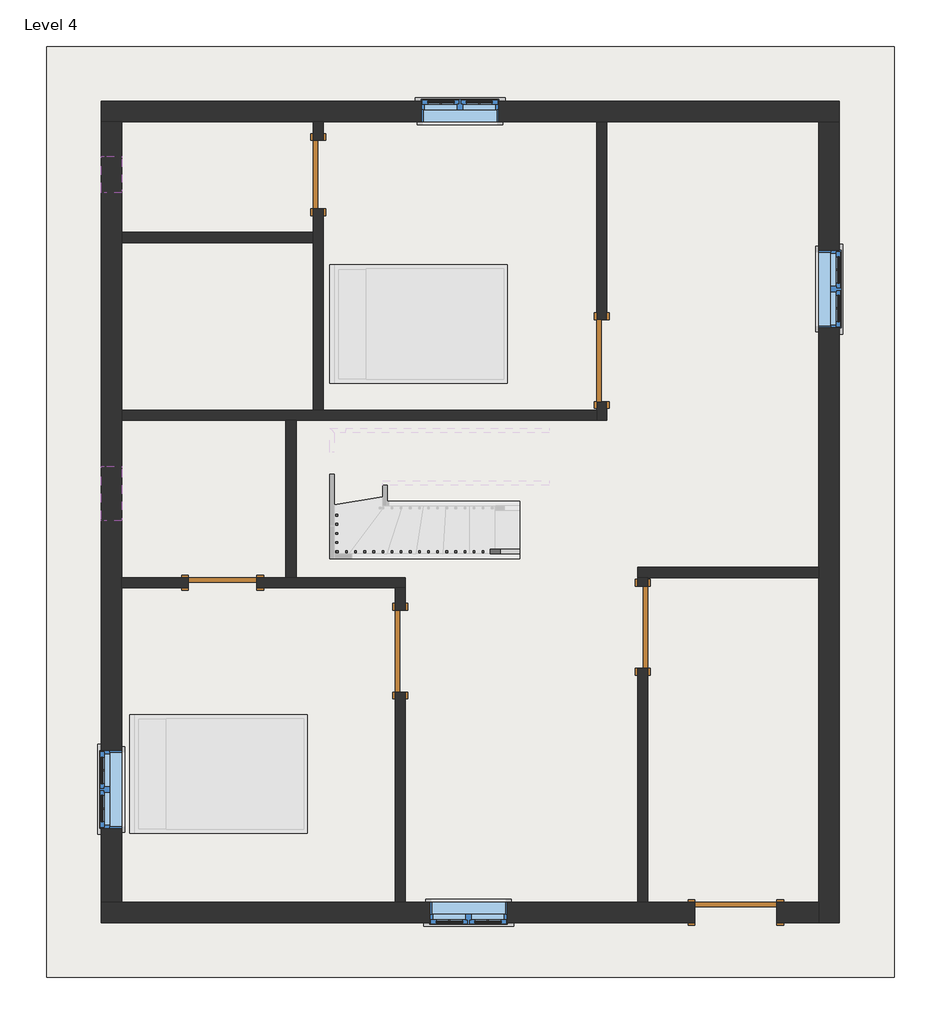
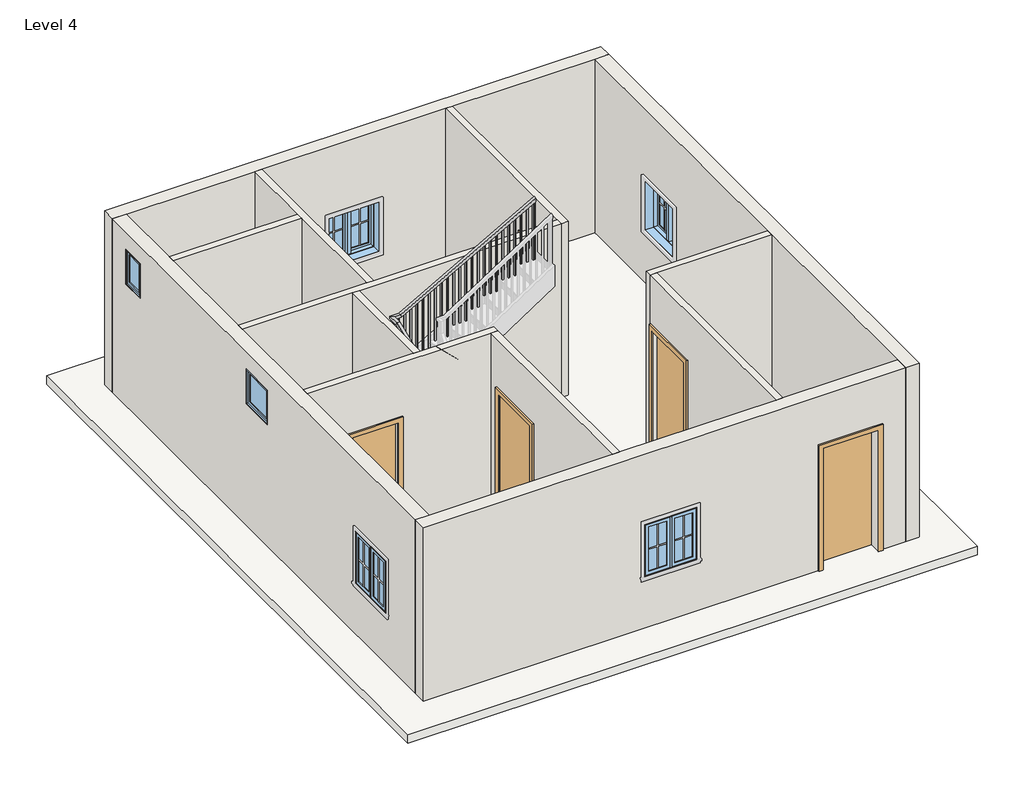
# One storey, part 1 of 2: 13 walls, 6 doors, 6 windows, 1 railing, 1 roof.
"""IFC4 building model written with IfcOpenShell, lengths in millimetres."""

from ifc_helpers import new_model, si_unit, frame, origin, place, context, project, spatial, polyline, outline, extrude, faceted_brep, transform, mapped, element, save
from components import door_d8f5dbb5, door_f2b275c1, door_305aa2a5, door_e5f9f3c4, door_0ca8825f, window_aa618e30, window_80340324, window_339605e1

model = new_model("IFC4")

# Units and contexts
model_context = context("Model", 3, world=origin())
ifc_project = project(units=[si_unit("LENGTHUNIT", "METRE", prefix="MILLI")], contexts=[model_context])

# Site, building, storey
site = spatial("IfcSite", under=ifc_project)
building = spatial("IfcBuilding", under=site)
storey = spatial("IfcBuildingStorey", under=building, Name="Level 4", Elevation=6400.8)

# Doors
placement = place(None, origin())
door_shape = door_d8f5dbb5(model_context)
element("IfcDoor", 1, ObjectType="Single-Flush : 30\" x 80\"", at=placement, inside=storey, context=model_context, shape_type="MappedRepresentation", body=[
    mapped(door_shape, transform((-2510.1648498, 3958.5558073, 6400.8), x_axis=(0.0, 1.0, 0.0), y_axis=(-1.0, 0.0, 0.0), z_axis=(0.0, 0.0, 1.0))),
])
door_2_shape = door_f2b275c1(model_context)
element("IfcDoor", 2, ObjectType="Single-Flush : 30\" x 80\"", at=placement, inside=storey, context=model_context, shape_type="MappedRepresentation", body=[
    mapped(door_2_shape, transform((-3576.9648498, -592.8066927, 6400.8), x_axis=(-1.0, 0.0, 0.0), y_axis=(0.0, -1.0, 0.0), z_axis=(0.0, 0.0, 1.0))),
])
door_3_shape = door_305aa2a5(model_context)
element("IfcDoor", 3, ObjectType="Single-Flush : 36\" x 84\"", at=placement, inside=storey, context=model_context, shape_type="MappedRepresentation", body=[
    mapped(door_3_shape, transform((652.1351502, 1883.6933073, 6400.8), x_axis=(0.0, -1.0, 0.0), y_axis=(1.0, 0.0, 0.0), z_axis=(0.0, 0.0, 1.0))),
])
element("IfcDoor", 4, ObjectType="Single-Flush : 36\" x 84\"", at=placement, inside=storey, context=model_context, shape_type="MappedRepresentation", body=[
    mapped(door_3_shape, transform((1109.3351502, -1088.1066927, 6400.8), x_axis=(0.0, 1.0, 0.0), y_axis=(-1.0, 0.0, 0.0), z_axis=(0.0, 0.0, 1.0))),
])
door_4_shape = door_e5f9f3c4(model_context)
element("IfcDoor", 5, ObjectType="Single-Flush : 36\" x 84\"", at=placement, inside=storey, context=model_context, shape_type="MappedRepresentation", body=[
    mapped(door_4_shape, transform((-1595.7648498, -1354.8066927, 6400.8), x_axis=(0.0, 1.0, 0.0), y_axis=(-1.0, 0.0, 0.0), z_axis=(0.0, 0.0, 1.0))),
])
door_5_shape = door_0ca8825f(model_context)
element("IfcDoor", 6, ObjectType="Single-Flush : 36\" x 84\"", at=placement, inside=storey, context=model_context, shape_type="MappedRepresentation", body=[
    mapped(door_5_shape, transform((2147.5601502, -4269.4566927, 6400.8), x_axis=(1.0, 0.0, 0.0), y_axis=(0.0, 1.0, 0.0), z_axis=(0.0, 0.0, 1.0))),
])

# Railing
element("IfcRailing", 7, ObjectType="Handrail - Rectangular", at=placement, inside=storey, context=model_context, shape_type="SolidModel", body=[
    faceted_brep([(-264.8831579, -271.8029286, 7484.5333333), (-264.8831579, -271.8029286, 7426.9518622), (-264.8831579, -221.0029286, 7426.9518622), (-264.8831579, -221.0029286, 7484.5333333), (-2203.3957557, -271.8029286, 8519.066441), (-2216.1029055, -271.8029286, 8468.266441), (-2216.1029055, -221.0029286, 8468.266441), (-2203.3957557, -221.0029286, 8519.066441), (-2328.8610857, -271.8029286, 8519.066441), (-2328.8610857, -271.8029286, 8468.266441), (-2278.0610857, -221.0029286, 8468.266441), (-2278.0610857, -221.0029286, 8519.066441), (-2328.8610857, -117.3180853, 8519.066441), (-2328.8610857, -107.2249429, 8468.266441), (-2278.0610857, -107.2249429, 8468.266441), (-2278.0610857, -117.3180853, 8519.066441), (-2328.8610857, 889.2076495, 8935.4648193), (-2328.8610857, 899.300792, 8884.6648193), (-2278.0610857, 899.300792, 8884.6648193), (-2278.0610857, 889.2076495, 8935.4648193), (-2328.8610857, 1080.0895433, 8935.4648193), (-2328.8610857, 1080.0895433, 8884.6648193), (-2278.0610857, 1029.2895433, 8884.6648193), (-2278.0610857, 1029.2895433, 8935.4648193), (-2181.3423106, 1080.0895433, 8935.4648193), (-2168.0744201, 1080.0895433, 8884.6648193), (-2168.0744201, 1029.2895433, 8884.6648193), (-2181.3423106, 1029.2895433, 8935.4648193), (63.4034409, 1080.0895433, 10193.8666667), (63.4034409, 1029.2895433, 10193.8666667), (63.4034409, 1029.2895433, 10135.6287027), (63.4034409, 1080.0895433, 10135.6287027)], [[[0, 1, 2, 3]], [[1, 0, 4, 5]], [[2, 1, 5, 6]], [[3, 2, 6, 7]], [[0, 3, 7, 4]], [[5, 4, 8, 9]], [[6, 5, 9, 10]], [[7, 6, 10, 11]], [[4, 7, 11, 8]], [[9, 8, 12, 13]], [[10, 9, 13, 14]], [[11, 10, 14, 15]], [[8, 11, 15, 12]], [[13, 12, 16, 17]], [[14, 13, 17, 18]], [[15, 14, 18, 19]], [[12, 15, 19, 16]], [[17, 16, 20, 21]], [[18, 17, 21, 22]], [[19, 18, 22, 23]], [[16, 19, 23, 20]], [[21, 20, 24, 25]], [[22, 21, 25, 26]], [[23, 22, 26, 27]], [[20, 23, 27, 24]], [[28, 29, 30, 31]], [[25, 24, 28, 31]], [[26, 25, 31, 30]], [[27, 26, 30, 29]], [[24, 27, 29, 28]]]),
    extrude(outline(polyline([(10113.4348603, 23.8139143), (9110.1333333, 23.8139143), (9110.1333333, 42.8639143), (10124.1142681, 42.8639143), (10113.4348603, 23.8139143)])), frame((0.0, 1045.1645433, 0.0), z_axis=(0.0, 1.0, 0.0), x_axis=(0.0, 0.0, 1.0)), (0.0, 0.0, 1.0), 19.05),
    extrude(outline(polyline([(10056.478019, -77.7860857), (9110.1333333, -77.7860857), (9110.1333333, -58.7360857), (10067.1574267, -58.7360857), (10056.478019, -77.7860857)])), frame((0.0, 1045.1645433, 0.0), z_axis=(0.0, 1.0, 0.0), x_axis=(0.0, 0.0, 1.0)), (0.0, 0.0, 1.0), 19.05),
    extrude(outline(polyline([(9999.5211776, -179.3860857), (9110.1333333, -179.3860857), (9110.1333333, -160.3360857), (10010.2005853, -160.3360857), (9999.5211776, -179.3860857)])), frame((0.0, 1045.1645433, 0.0), z_axis=(0.0, 1.0, 0.0), x_axis=(0.0, 0.0, 1.0)), (0.0, 0.0, 1.0), 19.05),
    extrude(outline(polyline([(9942.5643362, -280.9860857), (8940.8, -280.9860857), (8940.8, -261.9360857), (9953.243744, -261.9360857), (9942.5643362, -280.9860857)])), frame((0.0, 1045.1645433, 0.0), z_axis=(0.0, 1.0, 0.0), x_axis=(0.0, 0.0, 1.0)), (0.0, 0.0, 1.0), 19.05),
    extrude(outline(polyline([(9885.6074948, -382.5860857), (8940.8, -382.5860857), (8940.8, -363.5360857), (9896.2869026, -363.5360857), (9885.6074948, -382.5860857)])), frame((0.0, 1045.1645433, 0.0), z_axis=(0.0, 1.0, 0.0), x_axis=(0.0, 0.0, 1.0)), (0.0, 0.0, 1.0), 19.05),
    extrude(outline(polyline([(9828.6506535, -484.1860857), (8940.8, -484.1860857), (8940.8, -465.1360857), (9839.3300612, -465.1360857), (9828.6506535, -484.1860857)])), frame((0.0, 1045.1645433, 0.0), z_axis=(0.0, 1.0, 0.0), x_axis=(0.0, 0.0, 1.0)), (0.0, 0.0, 1.0), 19.05),
    extrude(outline(polyline([(9771.6938121, -585.7860857), (8771.4666667, -585.7860857), (8771.4666667, -566.7360857), (9782.3732198, -566.7360857), (9771.6938121, -585.7860857)])), frame((0.0, 1045.1645433, 0.0), z_axis=(0.0, 1.0, 0.0), x_axis=(0.0, 0.0, 1.0)), (0.0, 0.0, 1.0), 19.05),
    extrude(outline(polyline([(9714.7369707, -687.3860857), (8771.4666667, -687.3860857), (8771.4666667, -668.3360857), (9725.4163785, -668.3360857), (9714.7369707, -687.3860857)])), frame((0.0, 1045.1645433, 0.0), z_axis=(0.0, 1.0, 0.0), x_axis=(0.0, 0.0, 1.0)), (0.0, 0.0, 1.0), 19.05),
    extrude(outline(polyline([(9657.7801293, -788.9860857), (8771.4666667, -788.9860857), (8771.4666667, -769.9360857), (9668.4595371, -769.9360857), (9657.7801293, -788.9860857)])), frame((0.0, 1045.1645433, 0.0), z_axis=(0.0, 1.0, 0.0), x_axis=(0.0, 0.0, 1.0)), (0.0, 0.0, 1.0), 19.05),
    extrude(outline(polyline([(9600.823288, -890.5860857), (8602.1333333, -890.5860857), (8602.1333333, -871.5360857), (9611.5026957, -871.5360857), (9600.823288, -890.5860857)])), frame((0.0, 1045.1645433, 0.0), z_axis=(0.0, 1.0, 0.0), x_axis=(0.0, 0.0, 1.0)), (0.0, 0.0, 1.0), 19.05),
    extrude(outline(polyline([(9543.8664466, -992.1860857), (8602.1333333, -992.1860857), (8602.1333333, -973.1360857), (9554.5458543, -973.1360857), (9543.8664466, -992.1860857)])), frame((0.0, 1045.1645433, 0.0), z_axis=(0.0, 1.0, 0.0), x_axis=(0.0, 0.0, 1.0)), (0.0, 0.0, 1.0), 19.05),
    extrude(outline(polyline([(9486.9096052, -1093.7860857), (8432.8, -1093.7860857), (8432.8, -1074.7360857), (9497.589013, -1074.7360857), (9486.9096052, -1093.7860857)])), frame((0.0, 1045.1645433, 0.0), z_axis=(0.0, 1.0, 0.0), x_axis=(0.0, 0.0, 1.0)), (0.0, 0.0, 1.0), 19.05),
    extrude(outline(polyline([(9429.9527638, -1195.3860857), (8432.8, -1195.3860857), (8432.8, -1176.3360857), (9440.6321716, -1176.3360857), (9429.9527638, -1195.3860857)])), frame((0.0, 1045.1645433, 0.0), z_axis=(0.0, 1.0, 0.0), x_axis=(0.0, 0.0, 1.0)), (0.0, 0.0, 1.0), 19.05),
    extrude(outline(polyline([(9372.9959225, -1296.9860857), (8432.8, -1296.9860857), (8432.8, -1277.9360857), (9383.6753302, -1277.9360857), (9372.9959225, -1296.9860857)])), frame((0.0, 1045.1645433, 0.0), z_axis=(0.0, 1.0, 0.0), x_axis=(0.0, 0.0, 1.0)), (0.0, 0.0, 1.0), 19.05),
    extrude(outline(polyline([(9316.0390811, -1398.5860857), (8263.4666667, -1398.5860857), (8263.4666667, -1379.5360857), (9326.7184889, -1379.5360857), (9316.0390811, -1398.5860857)])), frame((0.0, 1045.1645433, 0.0), z_axis=(0.0, 1.0, 0.0), x_axis=(0.0, 0.0, 1.0)), (0.0, 0.0, 1.0), 19.05),
    extrude(outline(polyline([(9259.0822397, -1500.1860857), (8263.4666667, -1500.1860857), (8263.4666667, -1481.1360857), (9269.7616475, -1481.1360857), (9259.0822397, -1500.1860857)])), frame((0.0, 1045.1645433, 0.0), z_axis=(0.0, 1.0, 0.0), x_axis=(0.0, 0.0, 1.0)), (0.0, 0.0, 1.0), 19.05),
    extrude(outline(polyline([(9202.1253983, -1601.7860857), (8263.4666667, -1601.7860857), (8263.4666667, -1582.7360857), (9212.8048061, -1582.7360857), (9202.1253983, -1601.7860857)])), frame((0.0, 1045.1645433, 0.0), z_axis=(0.0, 1.0, 0.0), x_axis=(0.0, 0.0, 1.0)), (0.0, 0.0, 1.0), 19.05),
    extrude(outline(polyline([(9145.168557, -1703.3860857), (8094.1333333, -1703.3860857), (8094.1333333, -1684.3360857), (9155.8479647, -1684.3360857), (9145.168557, -1703.3860857)])), frame((0.0, 1045.1645433, 0.0), z_axis=(0.0, 1.0, 0.0), x_axis=(0.0, 0.0, 1.0)), (0.0, 0.0, 1.0), 19.05),
    extrude(outline(polyline([(9088.2117156, -1804.9860857), (8094.1333333, -1804.9860857), (8094.1333333, -1785.9360857), (9098.8911234, -1785.9360857), (9088.2117156, -1804.9860857)])), frame((0.0, 1045.1645433, 0.0), z_axis=(0.0, 1.0, 0.0), x_axis=(0.0, 0.0, 1.0)), (0.0, 0.0, 1.0), 19.05),
    extrude(outline(polyline([(9031.2548742, -1906.5860857), (8094.1333333, -1906.5860857), (8094.1333333, -1887.5360857), (9041.934282, -1887.5360857), (9031.2548742, -1906.5860857)])), frame((0.0, 1045.1645433, 0.0), z_axis=(0.0, 1.0, 0.0), x_axis=(0.0, 0.0, 1.0)), (0.0, 0.0, 1.0), 19.05),
    extrude(outline(polyline([(8974.2980329, -2008.1860857), (8094.1333333, -2008.1860857), (8094.1333333, -1989.1360857), (8984.9774406, -1989.1360857), (8974.2980329, -2008.1860857)])), frame((0.0, 1045.1645433, 0.0), z_axis=(0.0, 1.0, 0.0), x_axis=(0.0, 0.0, 1.0)), (0.0, 0.0, 1.0), 19.05),
    extrude(outline(polyline([(8917.3411915, -2109.7860857), (7924.8, -2109.7860857), (7924.8, -2090.7360857), (8928.0205992, -2090.7360857), (8917.3411915, -2109.7860857)])), frame((0.0, 1045.1645433, 0.0), z_axis=(0.0, 1.0, 0.0), x_axis=(0.0, 0.0, 1.0)), (0.0, 0.0, 1.0), 19.05),
    extrude(outline(polyline([(-2211.3860857, 1064.2145433), (-2192.3360857, 1064.2145433), (-2192.3360857, 1045.1645433), (-2211.3860857, 1045.1645433), (-2211.3860857, 1064.2145433)])), frame((0.0, 0.0, 7924.8), z_axis=(0.0, 0.0, 1.0), x_axis=(1.0, 0.0, 0.0)), (0.0, 0.0, 1.0), 959.8648193),
    extrude(outline(polyline([(-2312.9860857, 963.2720714), (-2312.9860857, 982.3220714), (-2293.9360857, 982.3220714), (-2293.9360857, 963.2720714), (-2312.9860857, 963.2720714)])), frame((0.0, 0.0, 7924.8), z_axis=(0.0, 0.0, 1.0), x_axis=(1.0, 0.0, 0.0)), (0.0, 0.0, 1.0), 959.8648193),
    extrude(outline(polyline([(880.7220714, 8876.9788269), (880.7220714, 7924.8), (861.6720714, 7924.8), (861.6720714, 8869.0978669), (880.7220714, 8876.9788269)])), frame((-2312.9860857, 0.0, 0.0), z_axis=(1.0, 0.0, 0.0), x_axis=(0.0, 1.0, 0.0)), (0.0, 0.0, 1.0), 19.05),
    extrude(outline(polyline([(779.1220714, 8834.94704), (779.1220714, 7924.8), (760.0720714, 7924.8), (760.0720714, 8827.0660799), (779.1220714, 8834.94704)])), frame((-2312.9860857, 0.0, 0.0), z_axis=(1.0, 0.0, 0.0), x_axis=(0.0, 1.0, 0.0)), (0.0, 0.0, 1.0), 19.05),
    extrude(outline(polyline([(677.5220714, 8792.915253), (677.5220714, 7924.8), (658.4720714, 7924.8), (658.4720714, 8785.034293), (677.5220714, 8792.915253)])), frame((-2312.9860857, 0.0, 0.0), z_axis=(1.0, 0.0, 0.0), x_axis=(0.0, 1.0, 0.0)), (0.0, 0.0, 1.0), 19.05),
    extrude(outline(polyline([(575.9220714, 8750.8834661), (575.9220714, 7755.4666667), (556.8720714, 7755.4666667), (556.8720714, 8743.002506), (575.9220714, 8750.8834661)])), frame((-2312.9860857, 0.0, 0.0), z_axis=(1.0, 0.0, 0.0), x_axis=(0.0, 1.0, 0.0)), (0.0, 0.0, 1.0), 19.05),
    extrude(outline(polyline([(474.3220714, 8708.8516792), (474.3220714, 7755.4666667), (455.2720714, 7755.4666667), (455.2720714, 8700.9707191), (474.3220714, 8708.8516792)])), frame((-2312.9860857, 0.0, 0.0), z_axis=(1.0, 0.0, 0.0), x_axis=(0.0, 1.0, 0.0)), (0.0, 0.0, 1.0), 19.05),
    extrude(outline(polyline([(372.7220714, 8666.8198922), (372.7220714, 7755.4666667), (353.6720714, 7755.4666667), (353.6720714, 8658.9389322), (372.7220714, 8666.8198922)])), frame((-2312.9860857, 0.0, 0.0), z_axis=(1.0, 0.0, 0.0), x_axis=(0.0, 1.0, 0.0)), (0.0, 0.0, 1.0), 19.05),
    extrude(outline(polyline([(271.1220714, 8624.7881053), (271.1220714, 7755.4666667), (252.0720714, 7755.4666667), (252.0720714, 8616.9071452), (271.1220714, 8624.7881053)])), frame((-2312.9860857, 0.0, 0.0), z_axis=(1.0, 0.0, 0.0), x_axis=(0.0, 1.0, 0.0)), (0.0, 0.0, 1.0), 19.05),
    extrude(outline(polyline([(169.5220714, 8582.7563183), (169.5220714, 7586.1333333), (150.4720714, 7586.1333333), (150.4720714, 8574.8753583), (169.5220714, 8582.7563183)])), frame((-2312.9860857, 0.0, 0.0), z_axis=(1.0, 0.0, 0.0), x_axis=(0.0, 1.0, 0.0)), (0.0, 0.0, 1.0), 19.05),
    extrude(outline(polyline([(67.9220714, 8540.7245314), (67.9220714, 7586.1333333), (48.8720714, 7586.1333333), (48.8720714, 8532.8435714), (67.9220714, 8540.7245314)])), frame((-2312.9860857, 0.0, 0.0), z_axis=(1.0, 0.0, 0.0), x_axis=(0.0, 1.0, 0.0)), (0.0, 0.0, 1.0), 19.05),
    extrude(outline(polyline([(-33.6779286, 8498.6927445), (-33.6779286, 7586.1333333), (-52.7279286, 7586.1333333), (-52.7279286, 8490.8117844), (-33.6779286, 8498.6927445)])), frame((-2312.9860857, 0.0, 0.0), z_axis=(1.0, 0.0, 0.0), x_axis=(0.0, 1.0, 0.0)), (0.0, 0.0, 1.0), 19.05),
    extrude(outline(polyline([(-2312.9860857, -154.3279286), (-2312.9860857, -135.2779286), (-2293.9360857, -135.2779286), (-2293.9360857, -154.3279286), (-2312.9860857, -154.3279286)])), frame((0.0, 0.0, 7586.1333333), z_axis=(0.0, 0.0, 1.0), x_axis=(1.0, 0.0, 0.0)), (0.0, 0.0, 1.0), 882.1331077),
    extrude(outline(polyline([(-2287.3581579, -255.9279286), (-2306.4081579, -255.9279286), (-2306.4081579, -236.8779286), (-2287.3581579, -236.8779286), (-2287.3581579, -255.9279286)])), frame((0.0, 0.0, 7586.1333333), z_axis=(0.0, 0.0, 1.0), x_axis=(1.0, 0.0, 0.0)), (0.0, 0.0, 1.0), 882.1331077),
    extrude(outline(polyline([(8462.2387317, -2204.8081579), (7586.1333333, -2204.8081579), (7586.1333333, -2185.7581579), (8452.0722486, -2185.7581579), (8462.2387317, -2204.8081579)])), frame((0.0, -255.9279286, 0.0), z_axis=(0.0, 1.0, 0.0), x_axis=(0.0, 0.0, 1.0)), (0.0, 0.0, 1.0), 19.05),
    extrude(outline(polyline([(8408.0174882, -2103.2081579), (7416.8, -2103.2081579), (7416.8, -2084.1581579), (8397.851005, -2084.1581579), (8408.0174882, -2103.2081579)])), frame((0.0, -255.9279286, 0.0), z_axis=(0.0, 1.0, 0.0), x_axis=(0.0, 0.0, 1.0)), (0.0, 0.0, 1.0), 19.05),
    extrude(outline(polyline([(8353.7962446, -2001.6081579), (7416.8, -2001.6081579), (7416.8, -1982.5581579), (8343.6297614, -1982.5581579), (8353.7962446, -2001.6081579)])), frame((0.0, -255.9279286, 0.0), z_axis=(0.0, 1.0, 0.0), x_axis=(0.0, 0.0, 1.0)), (0.0, 0.0, 1.0), 19.05),
    extrude(outline(polyline([(8299.575001, -1900.0081579), (7416.8, -1900.0081579), (7416.8, -1880.9581579), (8289.4085178, -1880.9581579), (8299.575001, -1900.0081579)])), frame((0.0, -255.9279286, 0.0), z_axis=(0.0, 1.0, 0.0), x_axis=(0.0, 0.0, 1.0)), (0.0, 0.0, 1.0), 19.05),
    extrude(outline(polyline([(8245.3537574, -1798.4081579), (7416.8, -1798.4081579), (7416.8, -1779.3581579), (8235.1872743, -1779.3581579), (8245.3537574, -1798.4081579)])), frame((0.0, -255.9279286, 0.0), z_axis=(0.0, 1.0, 0.0), x_axis=(0.0, 0.0, 1.0)), (0.0, 0.0, 1.0), 19.05),
    extrude(outline(polyline([(8191.1325139, -1696.8081579), (7247.4666667, -1696.8081579), (7247.4666667, -1677.7581579), (8180.9660307, -1677.7581579), (8191.1325139, -1696.8081579)])), frame((0.0, -255.9279286, 0.0), z_axis=(0.0, 1.0, 0.0), x_axis=(0.0, 0.0, 1.0)), (0.0, 0.0, 1.0), 19.05),
    extrude(outline(polyline([(8136.9112703, -1595.2081579), (7247.4666667, -1595.2081579), (7247.4666667, -1576.1581579), (8126.7447871, -1576.1581579), (8136.9112703, -1595.2081579)])), frame((0.0, -255.9279286, 0.0), z_axis=(0.0, 1.0, 0.0), x_axis=(0.0, 0.0, 1.0)), (0.0, 0.0, 1.0), 19.05),
    extrude(outline(polyline([(8082.6900267, -1493.6081579), (7247.4666667, -1493.6081579), (7247.4666667, -1474.5581579), (8072.5235435, -1474.5581579), (8082.6900267, -1493.6081579)])), frame((0.0, -255.9279286, 0.0), z_axis=(0.0, 1.0, 0.0), x_axis=(0.0, 0.0, 1.0)), (0.0, 0.0, 1.0), 19.05),
    extrude(outline(polyline([(8028.4687831, -1392.0081579), (7078.1333333, -1392.0081579), (7078.1333333, -1372.9581579), (8018.3023, -1372.9581579), (8028.4687831, -1392.0081579)])), frame((0.0, -255.9279286, 0.0), z_axis=(0.0, 1.0, 0.0), x_axis=(0.0, 0.0, 1.0)), (0.0, 0.0, 1.0), 19.05),
    extrude(outline(polyline([(7974.2475396, -1290.4081579), (7078.1333333, -1290.4081579), (7078.1333333, -1271.3581579), (7964.0810564, -1271.3581579), (7974.2475396, -1290.4081579)])), frame((0.0, -255.9279286, 0.0), z_axis=(0.0, 1.0, 0.0), x_axis=(0.0, 0.0, 1.0)), (0.0, 0.0, 1.0), 19.05),
    extrude(outline(polyline([(7920.026296, -1188.8081579), (7078.1333333, -1188.8081579), (7078.1333333, -1169.7581579), (7909.8598128, -1169.7581579), (7920.026296, -1188.8081579)])), frame((0.0, -255.9279286, 0.0), z_axis=(0.0, 1.0, 0.0), x_axis=(0.0, 0.0, 1.0)), (0.0, 0.0, 1.0), 19.05),
    extrude(outline(polyline([(7865.8050524, -1087.2081579), (6908.8, -1087.2081579), (6908.8, -1068.1581579), (7855.6385692, -1068.1581579), (7865.8050524, -1087.2081579)])), frame((0.0, -255.9279286, 0.0), z_axis=(0.0, 1.0, 0.0), x_axis=(0.0, 0.0, 1.0)), (0.0, 0.0, 1.0), 19.05),
    extrude(outline(polyline([(7811.5838088, -985.6081579), (6908.8, -985.6081579), (6908.8, -966.5581579), (7801.4173257, -966.5581579), (7811.5838088, -985.6081579)])), frame((0.0, -255.9279286, 0.0), z_axis=(0.0, 1.0, 0.0), x_axis=(0.0, 0.0, 1.0)), (0.0, 0.0, 1.0), 19.05),
    extrude(outline(polyline([(7757.3625653, -884.0081579), (6908.8, -884.0081579), (6908.8, -864.9581579), (7747.1960821, -864.9581579), (7757.3625653, -884.0081579)])), frame((0.0, -255.9279286, 0.0), z_axis=(0.0, 1.0, 0.0), x_axis=(0.0, 0.0, 1.0)), (0.0, 0.0, 1.0), 19.05),
    extrude(outline(polyline([(7703.1413217, -782.4081579), (6739.4666667, -782.4081579), (6739.4666667, -763.3581579), (7692.9748385, -763.3581579), (7703.1413217, -782.4081579)])), frame((0.0, -255.9279286, 0.0), z_axis=(0.0, 1.0, 0.0), x_axis=(0.0, 0.0, 1.0)), (0.0, 0.0, 1.0), 19.05),
    extrude(outline(polyline([(7648.9200781, -680.8081579), (6739.4666667, -680.8081579), (6739.4666667, -661.7581579), (7638.7535949, -661.7581579), (7648.9200781, -680.8081579)])), frame((0.0, -255.9279286, 0.0), z_axis=(0.0, 1.0, 0.0), x_axis=(0.0, 0.0, 1.0)), (0.0, 0.0, 1.0), 19.05),
    extrude(outline(polyline([(7594.6988345, -579.2081579), (6739.4666667, -579.2081579), (6739.4666667, -560.1581579), (7584.5323514, -560.1581579), (7594.6988345, -579.2081579)])), frame((0.0, -255.9279286, 0.0), z_axis=(0.0, 1.0, 0.0), x_axis=(0.0, 0.0, 1.0)), (0.0, 0.0, 1.0), 19.05),
    extrude(outline(polyline([(7540.477591, -477.6081579), (6570.1333333, -477.6081579), (6570.1333333, -458.5581579), (7530.3111078, -458.5581579), (7540.477591, -477.6081579)])), frame((0.0, -255.9279286, 0.0), z_axis=(0.0, 1.0, 0.0), x_axis=(0.0, 0.0, 1.0)), (0.0, 0.0, 1.0), 19.05),
    extrude(outline(polyline([(7486.2563474, -376.0081579), (6570.1333333, -376.0081579), (6570.1333333, -356.9581579), (7476.0898642, -356.9581579), (7486.2563474, -376.0081579)])), frame((0.0, -255.9279286, 0.0), z_axis=(0.0, 1.0, 0.0), x_axis=(0.0, 0.0, 1.0)), (0.0, 0.0, 1.0), 19.05),
    extrude(outline(polyline([(-2312.9860857, 1045.1645433), (-2312.9860857, 1064.2145433), (-2293.9360857, 1064.2145433), (-2293.9360857, 1045.1645433), (-2312.9860857, 1045.1645433)])), frame((0.0, 0.0, 7924.8), z_axis=(0.0, 0.0, 1.0), x_axis=(1.0, 0.0, 0.0)), (0.0, 0.0, 1.0), 959.8648193),
    extrude(outline(polyline([(-2293.9360857, -255.9279286), (-2312.9860857, -255.9279286), (-2312.9860857, -236.8779286), (-2293.9360857, -236.8779286), (-2293.9360857, -255.9279286)])), frame((0.0, 0.0, 7586.1333333), z_axis=(0.0, 0.0, 1.0), x_axis=(1.0, 0.0, 0.0)), (0.0, 0.0, 1.0), 882.1331077),
    extrude(outline(polyline([(10124.949295, 44.3534409), (9110.1333333, 44.3534409), (9110.1333333, 63.4034409), (10135.6287027, 63.4034409), (10124.949295, 44.3534409)])), frame((0.0, 1045.1645433, 0.0), z_axis=(0.0, 1.0, 0.0), x_axis=(0.0, 0.0, 1.0)), (0.0, 0.0, 1.0), 19.05),
    extrude(outline(polyline([(7437.1183454, -283.9331579), (6570.1333333, -283.9331579), (6570.1333333, -264.8831579), (7426.9518622, -264.8831579), (7437.1183454, -283.9331579)])), frame((0.0, -255.9279286, 0.0), z_axis=(0.0, 1.0, 0.0), x_axis=(0.0, 0.0, 1.0)), (0.0, 0.0, 1.0), 19.05),
])

# Roof
element("IfcRoof", 8, ObjectType="Generic - 12\"", at=placement, inside=storey, context=model_context, shape_type="SweptSolid", body=[
    extrude(outline(polyline([(-5539.1148498, 5385.7183073), (3909.6851502, 5385.7183073), (3909.6851502, -4993.3566927), (-5539.1148498, -4993.3566927), (-5539.1148498, 5385.7183073)])), frame((0.0, 0.0, 6248.4), z_axis=(0.0, 0.0, 1.0), x_axis=(1.0, 0.0, 0.0)), (0.0, 0.0, 1.0), 152.4),
])

# Walls
element("IfcWall", 9, ObjectType="WALL4.5\"", at=placement, inside=storey, context=model_context, shape_type="SweptSolid", body=[
    extrude(outline(polyline([(-2567.3148498, 3198.1433073), (-4700.9148498, 3198.1433073), (-4700.9148498, 3312.4433073), (-2567.3148498, 3312.4433073), (-2567.3148498, 3198.1433073)])), frame((0.0, 0.0, 6400.8), z_axis=(0.0, 0.0, 1.0), x_axis=(1.0, 0.0, 0.0)), (0.0, 0.0, 1.0), 3048.0),
])
element("IfcWall", 10, ObjectType="WALL4.5\"", at=placement, inside=storey, context=model_context, shape_type="Brep", body=[
    faceted_brep([(-2567.3148498, 4547.5183073, 6400.8), (-2567.3148498, 4339.5558073, 6400.8), (-2567.3148498, 4339.5558073, 8432.8), (-2567.3148498, 3577.5558073, 8432.8), (-2567.3148498, 3577.5558073, 6400.8), (-2567.3148498, 3312.4433073, 6400.8), (-2567.3148498, 3198.1433073, 6400.8), (-2567.3148498, 1331.2433073, 6400.8), (-2567.3148498, 1331.2433073, 9448.8), (-2567.3148498, 3198.1433073, 9448.8), (-2567.3148498, 3312.4433073, 9448.8), (-2567.3148498, 4547.5183073, 9448.8), (-2453.0148498, 4339.5558073, 8432.8), (-2453.0148498, 4339.5558073, 6400.8), (-2453.0148498, 4547.5183073, 6400.8), (-2453.0148498, 4547.5183073, 9448.8), (-2453.0148498, 1331.2433073, 9448.8), (-2453.0148498, 1331.2433073, 6400.8), (-2453.0148498, 3577.5558073, 6400.8), (-2453.0148498, 3577.5558073, 8432.8)], [[[0, 1, 2, 3, 4, 5, 6, 7, 8, 9, 10, 11]], [[12, 13, 14, 15, 16, 17, 18, 19]], [[18, 17, 7, 6, 5, 4]], [[14, 13, 1, 0]], [[0, 11, 15, 14]], [[8, 7, 17, 16]], [[2, 1, 13, 12]], [[3, 2, 12, 19]], [[4, 3, 19, 18]], [[11, 10, 9, 8, 16, 15]]]),
])
element("IfcWall", 11, ObjectType="WALL4.5\"", at=placement, inside=storey, context=model_context, shape_type="Brep", body=[
    faceted_brep([(594.9851502, 1426.4933073, 8534.4), (594.9851502, 1426.4933073, 6400.8), (594.9851502, 1331.2433073, 6400.8), (594.9851502, 1216.9433073, 6400.8), (594.9851502, 1216.9433073, 9448.8), (594.9851502, 1331.2433073, 9448.8), (594.9851502, 4547.5183073, 9448.8), (594.9851502, 4547.5183073, 6400.8), (594.9851502, 2340.8933073, 6400.8), (594.9851502, 2340.8933073, 8534.4), (709.2851502, 1216.9433073, 6400.8), (709.2851502, 1426.4933073, 6400.8), (709.2851502, 1426.4933073, 8534.4), (709.2851502, 2340.8933073, 8534.4), (709.2851502, 2340.8933073, 6400.8), (709.2851502, 4547.5183073, 6400.8), (709.2851502, 4547.5183073, 9448.8), (709.2851502, 1216.9433073, 9448.8)], [[[0, 1, 2, 3, 4, 5, 6, 7, 8, 9]], [[10, 11, 12, 13, 14, 15, 16, 17]], [[8, 7, 15, 14]], [[3, 2, 1, 11, 10]], [[7, 6, 16, 15]], [[4, 3, 10, 17]], [[12, 11, 1, 0]], [[13, 12, 0, 9]], [[14, 13, 9, 8]], [[6, 5, 4, 17, 16]]]),
])
element("IfcWall", 12, ObjectType="WALL4.5\"", at=placement, inside=storey, context=model_context, shape_type="Brep", body=[
    faceted_brep([(-4700.9148498, 1216.9433073, 6400.8), (-2872.1148498, 1216.9433073, 6400.8), (-2757.8148498, 1216.9433073, 6400.8), (594.9851502, 1216.9433073, 6400.8), (594.9851502, 1216.9433073, 9448.8), (-2757.8148498, 1216.9433073, 9448.8), (-2872.1148498, 1216.9433073, 9448.8), (-4700.9148498, 1216.9433073, 9448.8), (-4700.9148498, 1331.2433073, 6400.8), (-4700.9148498, 1331.2433073, 9448.8), (-2567.3148498, 1331.2433073, 9448.8), (-2453.0148498, 1331.2433073, 9448.8), (594.9851502, 1331.2433073, 9448.8), (594.9851502, 1331.2433073, 6400.8), (-2453.0148498, 1331.2433073, 6400.8), (-2567.3148498, 1331.2433073, 6400.8)], [[[0, 1, 2, 3, 4, 5, 6, 7]], [[8, 9, 10, 11, 12, 13, 14, 15]], [[3, 2, 1, 0, 8, 15, 14, 13]], [[4, 3, 13, 12]], [[0, 7, 9, 8]], [[7, 6, 5, 4, 12, 11, 10, 9]]]),
])
element("IfcWall", 13, ObjectType="WALL4.5\"", at=placement, inside=storey, context=model_context, shape_type="SweptSolid", body=[
    extrude(outline(polyline([(-2872.1148498, -535.6566927), (-2872.1148498, 1216.9433073), (-2757.8148498, 1216.9433073), (-2757.8148498, -535.6566927), (-2872.1148498, -535.6566927)])), frame((0.0, 0.0, 6400.8), z_axis=(0.0, 0.0, 1.0), x_axis=(1.0, 0.0, 0.0)), (0.0, 0.0, 1.0), 3048.0),
])
element("IfcWall", 14, ObjectType="WALL4.5\"", at=placement, inside=storey, context=model_context, shape_type="Brep", body=[
    faceted_brep([(-4700.9148498, -649.9566927, 6400.8), (-3957.9648498, -649.9566927, 6400.8), (-3957.9648498, -649.9566927, 8432.8), (-3195.9648498, -649.9566927, 8432.8), (-3195.9648498, -649.9566927, 6400.8), (-1652.9148498, -649.9566927, 6400.8), (-1538.6148498, -649.9566927, 6400.8), (-1538.6148498, -649.9566927, 9448.8), (-1652.9148498, -649.9566927, 9448.8), (-4700.9148498, -649.9566927, 9448.8), (-3957.9648498, -535.6566927, 8432.8), (-3957.9648498, -535.6566927, 6400.8), (-4700.9148498, -535.6566927, 6400.8), (-4700.9148498, -535.6566927, 9448.8), (-2872.1148498, -535.6566927, 9448.8), (-2757.8148498, -535.6566927, 9448.8), (-1538.6148498, -535.6566927, 9448.8), (-1538.6148498, -535.6566927, 6400.8), (-2757.8148498, -535.6566927, 6400.8), (-2872.1148498, -535.6566927, 6400.8), (-3195.9648498, -535.6566927, 6400.8), (-3195.9648498, -535.6566927, 8432.8)], [[[0, 1, 2, 3, 4, 5, 6, 7, 8, 9]], [[10, 11, 12, 13, 14, 15, 16, 17, 18, 19, 20, 21]], [[12, 11, 1, 0]], [[20, 19, 18, 17, 6, 5, 4]], [[7, 6, 17, 16]], [[0, 9, 13, 12]], [[2, 1, 11, 10]], [[3, 2, 10, 21]], [[4, 3, 21, 20]], [[9, 8, 7, 16, 15, 14, 13]]]),
])
element("IfcWall", 15, ObjectType="WALL4.5\"", at=placement, inside=storey, context=model_context, shape_type="Brep", body=[
    faceted_brep([(3071.4851502, -421.3566927, 6400.8), (1052.1851502, -421.3566927, 6400.8), (1052.1851502, -421.3566927, 9448.8), (3071.4851502, -421.3566927, 9448.8), (3071.4851502, -535.6566927, 6400.8), (3071.4851502, -535.6566927, 9448.8), (1166.4851502, -535.6566927, 9448.8), (1052.1851502, -535.6566927, 9448.8), (1052.1851502, -535.6566927, 6400.8), (1166.4851502, -535.6566927, 6400.8)], [[[0, 1, 2, 3]], [[4, 5, 6, 7, 8, 9]], [[1, 0, 4, 9, 8]], [[0, 3, 5, 4]], [[2, 1, 8, 7]], [[3, 2, 7, 6, 5]]]),
])
element("IfcWall", 16, ObjectType="WALL4.5\"", at=placement, inside=storey, context=model_context, shape_type="SweptSolid", body=[
    extrude(outline(polyline([(-535.6566927, 6400.8), (-630.9066927, 6400.8), (-630.9066927, 8534.4), (-1545.3066927, 8534.4), (-1545.3066927, 6400.8), (-4155.1566927, 6400.8), (-4155.1566927, 9448.8), (-535.6566927, 9448.8), (-535.6566927, 6400.8)])), frame((1052.1851502, 0.0, 0.0), z_axis=(1.0, 0.0, 0.0), x_axis=(0.0, 1.0, 0.0)), (0.0, 0.0, 1.0), 114.3),
])
element("IfcWall", 17, ObjectType="WALL4.5\"", at=placement, inside=storey, context=model_context, shape_type="SweptSolid", body=[
    extrude(outline(polyline([(-649.9566927, 6400.8), (-897.6066927, 6400.8), (-897.6066927, 8534.4), (-1812.0066927, 8534.4), (-1812.0066927, 6400.8), (-4155.1566927, 6400.8), (-4155.1566927, 9448.8), (-649.9566927, 9448.8), (-649.9566927, 6400.8)])), frame((-1652.9148498, 0.0, 0.0), z_axis=(1.0, 0.0, 0.0), x_axis=(0.0, 1.0, 0.0)), (0.0, 0.0, 1.0), 114.3),
])
element("IfcWall", 18, ObjectType="WALL9\"", at=placement, inside=storey, context=model_context, shape_type="Brep", body=[
    faceted_brep([(-4929.5148498, 4547.5183073, 6400.8), (-4700.9148498, 4547.5183073, 6400.8), (-2567.3148498, 4547.5183073, 6400.8), (-2453.0148498, 4547.5183073, 6400.8), (594.9851502, 4547.5183073, 6400.8), (709.2851502, 4547.5183073, 6400.8), (3071.4851502, 4547.5183073, 6400.8), (3300.0851502, 4547.5183073, 6400.8), (3300.0851502, 4547.5183073, 9448.8), (3071.4851502, 4547.5183073, 9448.8), (709.2851502, 4547.5183073, 9448.8), (594.9851502, 4547.5183073, 9448.8), (-2453.0148498, 4547.5183073, 9448.8), (-2567.3148498, 4547.5183073, 9448.8), (-4700.9148498, 4547.5183073, 9448.8), (-4929.5148498, 4547.5183073, 9448.8), (-497.2148498, 4547.5183073, 8229.6), (-497.2148498, 4547.5183073, 7315.2), (-1360.8148498, 4547.5183073, 7315.2), (-1360.8148498, 4547.5183073, 8229.6), (-4929.5148498, 4776.1183073, 6400.8), (-4929.5148498, 4776.1183073, 9448.8), (3300.0851502, 4776.1183073, 9448.8), (3300.0851502, 4776.1183073, 6400.8), (-497.2148498, 4776.1183073, 8229.6), (-1360.8148498, 4776.1183073, 8229.6), (-1360.8148498, 4776.1183073, 7315.2), (-497.2148498, 4776.1183073, 7315.2)], [[[0, 1, 2, 3, 4, 5, 6, 7, 8, 9, 10, 11, 12, 13, 14, 15], [16, 17, 18, 19]], [[20, 21, 22, 23], [24, 25, 26, 27]], [[7, 6, 5, 4, 3, 2, 1, 0, 20, 23]], [[8, 7, 23, 22]], [[0, 15, 21, 20]], [[17, 16, 24, 27]], [[18, 17, 27, 26]], [[19, 18, 26, 25]], [[16, 19, 25, 24]], [[15, 14, 13, 12, 11, 10, 9, 8, 22, 21]]]),
])
element("IfcWall", 19, ObjectType="WALL9\"", at=placement, inside=storey, context=model_context, shape_type="Brep", body=[
    faceted_brep([(3071.4851502, 4547.5183073, 6400.8), (3071.4851502, -421.3566927, 6400.8), (3071.4851502, -535.6566927, 6400.8), (3071.4851502, -4155.1566927, 6400.8), (3071.4851502, -4383.7566927, 6400.8), (3071.4851502, -4383.7566927, 9448.8), (3071.4851502, -4155.1566927, 9448.8), (3071.4851502, -535.6566927, 9448.8), (3071.4851502, -421.3566927, 9448.8), (3071.4851502, 4547.5183073, 9448.8), (3071.4851502, 2248.8183073, 8229.6), (3071.4851502, 2248.8183073, 7315.2), (3071.4851502, 3112.4183073, 7315.2), (3071.4851502, 3112.4183073, 8229.6), (3300.0851502, 4547.5183073, 6400.8), (3300.0851502, 4547.5183073, 9448.8), (3300.0851502, -4383.7566927, 9448.8), (3300.0851502, -4383.7566927, 6400.8), (3300.0851502, 2248.8183073, 8229.6), (3300.0851502, 3112.4183073, 8229.6), (3300.0851502, 3112.4183073, 7315.2), (3300.0851502, 2248.8183073, 7315.2)], [[[0, 1, 2, 3, 4, 5, 6, 7, 8, 9], [10, 11, 12, 13]], [[14, 15, 16, 17], [18, 19, 20, 21]], [[4, 3, 2, 1, 0, 14, 17]], [[0, 9, 15, 14]], [[5, 4, 17, 16]], [[11, 10, 18, 21]], [[12, 11, 21, 20]], [[13, 12, 20, 19]], [[10, 13, 19, 18]], [[9, 8, 7, 6, 5, 16, 15]]]),
])
element("IfcWall", 20, ObjectType="WALL9\"", at=placement, inside=storey, context=model_context, shape_type="Brep", body=[
    faceted_brep([(3071.4851502, -4155.1566927, 6400.8), (2604.7601502, -4155.1566927, 6400.8), (2604.7601502, -4155.1566927, 8534.4), (1690.3601502, -4155.1566927, 8534.4), (1690.3601502, -4155.1566927, 6400.8), (1166.4851502, -4155.1566927, 6400.8), (1052.1851502, -4155.1566927, 6400.8), (-1538.6148498, -4155.1566927, 6400.8), (-1652.9148498, -4155.1566927, 6400.8), (-4700.9148498, -4155.1566927, 6400.8), (-4929.5148498, -4155.1566927, 6400.8), (-4929.5148498, -4155.1566927, 9448.8), (-4700.9148498, -4155.1566927, 9448.8), (-1652.9148498, -4155.1566927, 9448.8), (-1538.6148498, -4155.1566927, 9448.8), (1052.1851502, -4155.1566927, 9448.8), (1166.4851502, -4155.1566927, 9448.8), (3071.4851502, -4155.1566927, 9448.8), (-1265.5648498, -4155.1566927, 8229.6), (-1265.5648498, -4155.1566927, 7315.2), (-401.9648498, -4155.1566927, 7315.2), (-401.9648498, -4155.1566927, 8229.6), (2604.7601502, -4383.7566927, 8534.4), (2604.7601502, -4383.7566927, 6400.8), (3071.4851502, -4383.7566927, 6400.8), (3071.4851502, -4383.7566927, 9448.8), (-4929.5148498, -4383.7566927, 9448.8), (-4929.5148498, -4383.7566927, 6400.8), (1690.3601502, -4383.7566927, 6400.8), (1690.3601502, -4383.7566927, 8534.4), (-1265.5648498, -4383.7566927, 8229.6), (-401.9648498, -4383.7566927, 8229.6), (-401.9648498, -4383.7566927, 7315.2), (-1265.5648498, -4383.7566927, 7315.2)], [[[0, 1, 2, 3, 4, 5, 6, 7, 8, 9, 10, 11, 12, 13, 14, 15, 16, 17], [18, 19, 20, 21]], [[22, 23, 24, 25, 26, 27, 28, 29], [30, 31, 32, 33]], [[28, 27, 10, 9, 8, 7, 6, 5, 4]], [[24, 23, 1, 0]], [[0, 17, 25, 24]], [[11, 10, 27, 26]], [[19, 18, 30, 33]], [[20, 19, 33, 32]], [[21, 20, 32, 31]], [[18, 21, 31, 30]], [[17, 16, 15, 14, 13, 12, 11, 26, 25]], [[2, 1, 23, 22]], [[3, 2, 22, 29]], [[4, 3, 29, 28]]]),
])
element("IfcWall", 21, ObjectType="WALL9\"", at=placement, inside=storey, context=model_context, shape_type="Brep", body=[
    faceted_brep([(-4700.9148498, -4155.1566927, 6400.8), (-4700.9148498, -649.9566927, 6400.8), (-4700.9148498, -535.6566927, 6400.8), (-4700.9148498, 1216.9433073, 6400.8), (-4700.9148498, 1331.2433073, 6400.8), (-4700.9148498, 3198.1433073, 6400.8), (-4700.9148498, 3312.4433073, 6400.8), (-4700.9148498, 4547.5183073, 6400.8), (-4700.9148498, 4547.5183073, 9448.8), (-4700.9148498, 3312.4433073, 9448.8), (-4700.9148498, 3198.1433073, 9448.8), (-4700.9148498, 1331.2433073, 9448.8), (-4700.9148498, 1216.9433073, 9448.8), (-4700.9148498, -535.6566927, 9448.8), (-4700.9148498, -649.9566927, 9448.8), (-4700.9148498, -4155.1566927, 9448.8), (-4700.9148498, 4161.7558073, 9144.0), (-4700.9148498, 4161.7558073, 8534.4), (-4700.9148498, 3755.3558073, 8534.4), (-4700.9148498, 3755.3558073, 9144.0), (-4700.9148498, 705.7683073, 9144.0), (-4700.9148498, 705.7683073, 8534.4), (-4700.9148498, 96.1683073, 8534.4), (-4700.9148498, 96.1683073, 9144.0), (-4700.9148498, -2466.0566927, 8229.6), (-4700.9148498, -2466.0566927, 7315.2), (-4700.9148498, -3329.6566927, 7315.2), (-4700.9148498, -3329.6566927, 8229.6), (-4929.5148498, -4155.1566927, 6400.8), (-4929.5148498, -4155.1566927, 9448.8), (-4929.5148498, 4547.5183073, 9448.8), (-4929.5148498, 4547.5183073, 6400.8), (-4929.5148498, 4161.7558073, 9144.0), (-4929.5148498, 3755.3558073, 9144.0), (-4929.5148498, 3755.3558073, 8534.4), (-4929.5148498, 4161.7558073, 8534.4), (-4929.5148498, 705.7683073, 9144.0), (-4929.5148498, 96.1683073, 9144.0), (-4929.5148498, 96.1683073, 8534.4), (-4929.5148498, 705.7683073, 8534.4), (-4929.5148498, -2466.0566927, 8229.6), (-4929.5148498, -3329.6566927, 8229.6), (-4929.5148498, -3329.6566927, 7315.2), (-4929.5148498, -2466.0566927, 7315.2)], [[[0, 1, 2, 3, 4, 5, 6, 7, 8, 9, 10, 11, 12, 13, 14, 15], [16, 17, 18, 19], [20, 21, 22, 23], [24, 25, 26, 27]], [[28, 29, 30, 31], [32, 33, 34, 35], [36, 37, 38, 39], [40, 41, 42, 43]], [[7, 6, 5, 4, 3, 2, 1, 0, 28, 31]], [[8, 7, 31, 30]], [[0, 15, 29, 28]], [[17, 16, 32, 35]], [[18, 17, 35, 34]], [[19, 18, 34, 33]], [[16, 19, 33, 32]], [[21, 20, 36, 39]], [[22, 21, 39, 38]], [[23, 22, 38, 37]], [[20, 23, 37, 36]], [[25, 24, 40, 43]], [[26, 25, 43, 42]], [[27, 26, 42, 41]], [[24, 27, 41, 40]], [[15, 14, 13, 12, 11, 10, 9, 8, 30, 29]]]),
])

# Windows
window_shape = window_aa618e30(model_context)
element("IfcWindow", 22, ObjectType="Fixed : 16\" x 24\"", at=placement, inside=storey, context=model_context, shape_type="MappedRepresentation", body=[
    mapped(window_shape, transform((-4815.2148498, 3996.6558073, 7620.0), x_axis=(0.0, 1.0, 0.0), y_axis=(-1.0, 0.0, 0.0), z_axis=(0.0, 0.0, 1.0))),
])
window_2_shape = window_80340324(model_context)
element("IfcWindow", 23, ObjectType="Fixed : 24\" x 24\"", at=placement, inside=storey, context=model_context, shape_type="MappedRepresentation", body=[
    mapped(window_2_shape, transform((-4815.2148498, 439.0683073, 7620.0), x_axis=(0.0, 1.0, 0.0), y_axis=(-1.0, 0.0, 0.0), z_axis=(0.0, 0.0, 1.0))),
])
window_3_shape = window_339605e1(model_context)
element("IfcWindow", 24, ObjectType="Window-Casement-Double : 34\" x 36\"", at=placement, inside=storey, context=model_context, shape_type="MappedRepresentation", body=[
    mapped(window_3_shape, transform((-929.0148498, 4661.8183073, 6400.8), x_axis=(1.0, 0.0, 0.0), y_axis=(0.0, 1.0, 0.0), z_axis=(0.0, 0.0, 1.0))),
])
element("IfcWindow", 25, ObjectType="Window-Casement-Double : 34\" x 36\"", at=placement, inside=storey, context=model_context, shape_type="MappedRepresentation", body=[
    mapped(window_3_shape, transform((3185.7851502, 2680.6183073, 6400.8), x_axis=(0.0, -1.0, 0.0), y_axis=(1.0, 0.0, 0.0), z_axis=(0.0, 0.0, 1.0))),
])
element("IfcWindow", 26, ObjectType="Window-Casement-Double : 34\" x 36\"", at=placement, inside=storey, context=model_context, shape_type="MappedRepresentation", body=[
    mapped(window_3_shape, transform((-833.7648498, -4269.4566927, 6400.8), x_axis=(-1.0, 0.0, 0.0), y_axis=(0.0, -1.0, 0.0), z_axis=(0.0, 0.0, 1.0))),
])
element("IfcWindow", 27, ObjectType="Window-Casement-Double : 34\" x 36\"", at=placement, inside=storey, context=model_context, shape_type="MappedRepresentation", body=[
    mapped(window_3_shape, transform((-4815.2148498, -2897.8566927, 6400.8), x_axis=(0.0, 1.0, 0.0), y_axis=(-1.0, 0.0, 0.0), z_axis=(0.0, 0.0, 1.0))),
])

save(model, "model.ifc")

# Revit data of these elements
# Type "Single-Flush : 30\" x 80\""
#   Type Mark = "5"
#   Construction Type Id = "MDOOR"
#   Assembly Code = "C1020"
#   Analytic Construction = "Metal"
#   Thickness = 0' - 2"
#   Heat Transfer Coefficient (U) = 0.651978 BTU/(h·ft²·°F)
#   Height = 6' - 8"
#   Trim Projection Ext = 0' - 1"
#   Trim Projection Int = 0' - 1"
#   Trim Width = 0' - 3"
#   Width = 2' - 6"
#   Define Thermal Properties by = 1
#   Define Thermal Properties by = 1
#   Door Material = Door - Panel
#   Frame Material = Door - Frame
#   Visual Light Transmittance = 0
#   Solar Heat Gain Coefficient = 0
#   Function = (empty or 0)
#   Wall Closure = (empty or 0)
# Type "Single-Flush : 36\" x 84\""
#   Type Mark = "1"
#   Construction Type Id = "MDOOR"
#   Assembly Code = "C1020"
#   Analytic Construction = "Metal"
#   Thickness = 0' - 2"
#   Heat Transfer Coefficient (U) = 0.651978 BTU/(h·ft²·°F)
#   Height = 7' - 0"
#   Trim Projection Ext = 0' - 1"
#   Trim Projection Int = 0' - 1"
#   Trim Width = 0' - 3"
#   Width = 3' - 0"
#   Define Thermal Properties by = 1
#   Define Thermal Properties by = 1
#   Door Material = Door - Panel
#   Frame Material = Door - Frame
#   Visual Light Transmittance = 0
#   Solar Heat Gain Coefficient = 0
#   Function = (empty or 0)
#   Wall Closure = (empty or 0)
# Type "Handrail - Rectangular"
#   Assembly Code = "C2010400"
#   built-in parameter 1008612 = 0.0416667 (stored number, unit not read)
#   built-in parameter 1008611 = 0.0416667 (stored number, unit not read)
#   built-in parameter 1008609 = 0.333333 (stored number, unit not read)
#   built-in parameter 1008604 = 0.166667 (stored number, unit not read)
#   built-in parameter 1008603 = 0.166667 (stored number, unit not read)
#   Railing Height = 3' - 0"
#   built-in parameter 1008630 = 2
#   built-in parameter 1008610 = 2
#   built-in parameter 1008618 = Baluster - Square : 3/4"
# Type "Generic - 12\""
#   Assembly Code = "B1020"
#   Layers, outside or top first: 0' - 6" no material (function 1)
# Type "WALL4.5\""
#   Assembly Code = "B2010"
#   Layers, outside or top first: 0' - 4 1/2" no material (function 1)
# Type "WALL9\""
#   Assembly Code = "B2010"
#   Layers, outside or top first: 0' - 9" no material (function 1)
# Type "Fixed : 16\" x 24\""
#   Type Mark = "4"
#   Construction Type Id = "GSP4R"
#   Assembly Code = "B2020100"
#   Analytic Construction = "1/8 in Pilkington single glazing"
#   Visual Light Transmittance = 0.9
#   Solar Heat Gain Coefficient = 0.78
#   Heat Transfer Coefficient (U) = 0.6496 BTU/(h·ft²·°F)
#   Height = 2' - 0"
#   Default Sill Height = 3' - 0"
#   Width = 1' - 4"
#   Window Inset = 0' - 0 3/4"
#   Define Thermal Properties by = 1
#   Define Thermal Properties by = 1
#   Glass Pane Material = Glass
#   Sash Material = Sash
#   Wall Closure = (empty or 0)
# Type "Fixed : 24\" x 24\""
#   Type Mark = "3"
#   Construction Type Id = "GSP4R"
#   Assembly Code = "B2020100"
#   Analytic Construction = "1/8 in Pilkington single glazing"
#   Visual Light Transmittance = 0.9
#   Solar Heat Gain Coefficient = 0.78
#   Heat Transfer Coefficient (U) = 0.6496 BTU/(h·ft²·°F)
#   Height = 2' - 0"
#   Default Sill Height = 3' - 0"
#   Width = 2' - 0"
#   Window Inset = 0' - 0 3/4"
#   Define Thermal Properties by = 1
#   Define Thermal Properties by = 1
#   Glass Pane Material = Glass
#   Sash Material = Sash
#   Wall Closure = (empty or 0)
# Type "Window-Casement-Double : 34\" x 36\""
#   Type Mark = "14"
#   Fire Rating = "0.5h"
#   Assembly Code = "B2020100"
#   Analytic Construction = "Double glazing - domestic"
#   Frame Extension [instance default] = 0' - 0 1/4"
#   Window Inset [instance default] = 0' - 0"
#   Wall Thickness [instance default] = 0' - 6"
#   Interior Wall Closure [instance default] = 0' - 2 1/4"
#   Half Width = 1' - 5"
#   Visual Light Transmittance = 0.81
#   Thermal Resistance (R) = 1.8146 (h·ft²·°F)/BTU
#   Solar Heat Gain Coefficient = 0.76
#   Rough Width = 2' - 10 1/2"
#   Rough Height = 3' - 0 1/2"
#   Height = 3' - 0"
#   Heat Transfer Coefficient (U) = 0.5511 BTU/(h·ft²·°F)
#   Exterior Wall Closure [instance default] = 0' - 1 1/4"
#   Extension Jamb [instance default] = 0' - 2 1/4"
#   Default Sill Height = 3' - 0"
#   Width = 2' - 10"
#   Define Thermal Properties by = 0
#   Muntin Visibility = yes
#   Interior Trim Visibility [instance default] = yes
#   Exterior Trim Visibility [instance default] = yes
#   Extension Jamb Visibility [instance default] = yes
#   Interior Trim Material = Wood - Stained
#   Muntin Pattern = Muntin Pattern_2x2 : Muntin Pattern_2x2
#   Interior Trim = Trim-Window-Interior-Flat : Picture Frame
#   Interior Frame Material = Wood - Stained
#   Glass Panel Material = Glass
#   Exterior Trim Material = Clad - White
#   Exterior Trim = Trim-Window-Exterior-Flat : with Sill
#   Exterior Frame Material = Clad - White
#   Wall Closure = (empty or 0)
# Elements 1, 2 (IfcDoor, "Single-Flush : 30\" x 80\"")
#   Phase Created = New Construction
#   Materials on its faces: "Door - Frame", "Door - Panel"
# Elements 3, 4, 5, 6 (IfcDoor, "Single-Flush : 36\" x 84\"")
#   Phase Created = New Construction
#   Materials on its faces: "Door - Frame", "Door - Panel"
# Element 7 (IfcRailing, "Handrail - Rectangular")
#   Phase Created = New Construction
# Element 8 (IfcRoof, "Generic - 12\"")
#   built-in parameter 1001705 = 21 (stored number, unit not read)
#   built-in parameter 1001701 = -0.5 (stored number, unit not read)
#   built-in parameter 1001710 = 33615
#   Phase Created = New Construction
#   Materials on its faces: "Default Roof", "Wood - Stained"
# Elements 9, 10, 11, 12, 13, 14, 15, 16, 17 (IfcWall, "WALL4.5\"")
#   Top Offset = 0' - 0"
#   Base Offset = 0' - 0"
#   Unconnected Height = 10' - 0"
#   wall height = 10' - 0"
#   Phase Created = New Construction
#   Base Constraint = Level 4
#   Materials on its faces: "Default Wall"
# Elements 18, 19, 20, 21 (IfcWall, "WALL9\"")
#   Top Offset = 0' - 0"
#   Base Offset = 0' - 0"
#   Unconnected Height = 10' - 0"
#   wall height = 10' - 0"
#   Phase Created = New Construction
#   Base Constraint = Level 4
#   Materials on its faces: "Default Wall", "Wood - Stained"
# Element 22 (IfcWindow, "Fixed : 16\" x 24\"")
#   Mark = "16"
#   Phase Created = New Construction
#   Materials on its faces: "Sash", "Glass"
# Element 23 (IfcWindow, "Fixed : 24\" x 24\"")
#   Mark = "20"
#   Phase Created = New Construction
#   Materials on its faces: "Sash", "Glass"
# Element 24 (IfcWindow, "Window-Casement-Double : 34\" x 36\"")
#   Mark = "17"
#   Window Inset = 0' - 0"
#   Interior Wall Closure = 0' - 2 1/4"
#   Frame Extension = 0' - 0 1/4"
#   Exterior Wall Closure = 0' - 1 1/4"
#   Interior Trim Visibility = yes
#   Exterior Trim Visibility = yes
#   Phase Created = New Construction
#   Materials on its faces: "Wood - Stained", "Glass", "Clad - White"
# Element 25 (IfcWindow, "Window-Casement-Double : 34\" x 36\"")
#   Mark = "18"
#   Window Inset = 0' - 0"
#   Interior Wall Closure = 0' - 2 1/4"
#   Frame Extension = 0' - 0 1/4"
#   Exterior Wall Closure = 0' - 1 1/4"
#   Interior Trim Visibility = yes
#   Exterior Trim Visibility = yes
#   Phase Created = New Construction
#   Materials on its faces: "Wood - Stained", "Glass", "Clad - White"
# Element 26 (IfcWindow, "Window-Casement-Double : 34\" x 36\"")
#   Mark = "19"
#   Window Inset = 0' - 0"
#   Interior Wall Closure = 0' - 2 1/4"
#   Frame Extension = 0' - 0 1/4"
#   Exterior Wall Closure = 0' - 1 1/4"
#   Interior Trim Visibility = yes
#   Exterior Trim Visibility = yes
#   Phase Created = New Construction
#   Materials on its faces: "Wood - Stained", "Glass", "Clad - White"
# Element 27 (IfcWindow, "Window-Casement-Double : 34\" x 36\"")
#   Mark = "21"
#   Window Inset = 0' - 0"
#   Interior Wall Closure = 0' - 2 1/4"
#   Frame Extension = 0' - 0 1/4"
#   Exterior Wall Closure = 0' - 1 1/4"
#   Interior Trim Visibility = yes
#   Exterior Trim Visibility = yes
#   Phase Created = New Construction
#   Materials on its faces: "Wood - Stained", "Glass", "Clad - White"
# Materials
#   "Door - Panel": class "Wood", colour RGB 210 159 95, transparency 0, Cost = 0
#   "Door - Frame": colour RGB 118 70 51, transparency 0, Cost = 0
#   "Glass": class "Glass", colour RGB 0 128 192, transparency 0.75, Description = "Soda Lime Glass", Cost = 0
#   "Sash": class "Wood", colour RGB 224 178 126, transparency 0, Cost = 0
#   "Wood - Stained": class "Wood", colour RGB 224 178 126, transparency 0, Cost = 0
#   "Clad - White": class "Wood", colour RGB 242 242 238, transparency 0, Cost = 0
#   "Default Roof": colour RGB 88 101 114, transparency 0, Cost = 0
#   "Default Wall": colour RGB 128 128 128, transparency 0, Cost = 0
